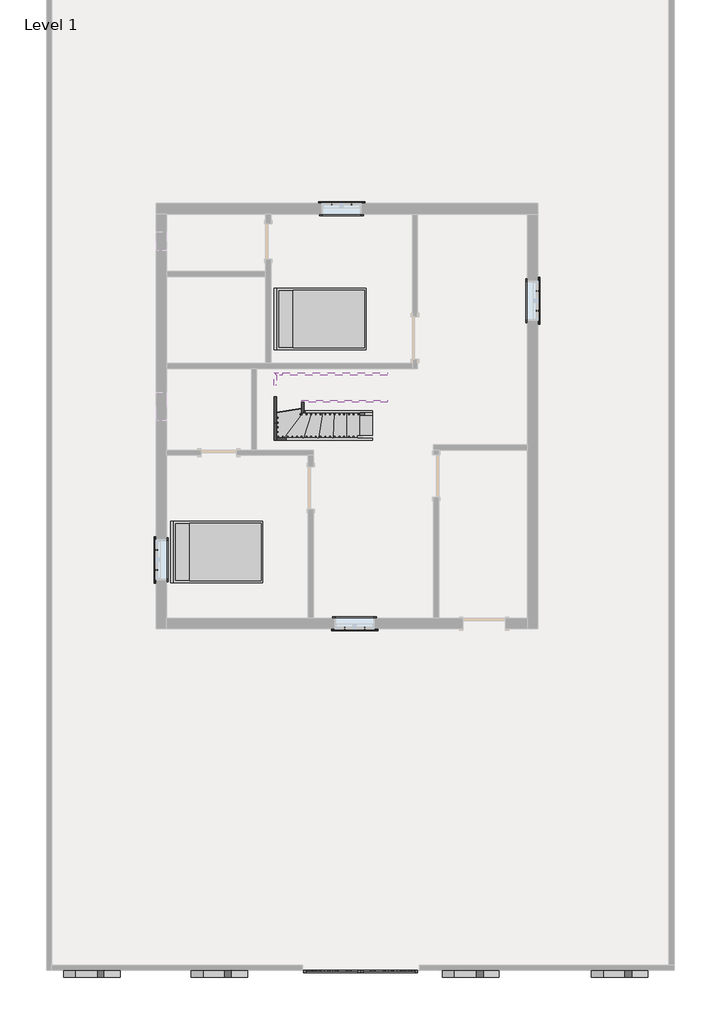
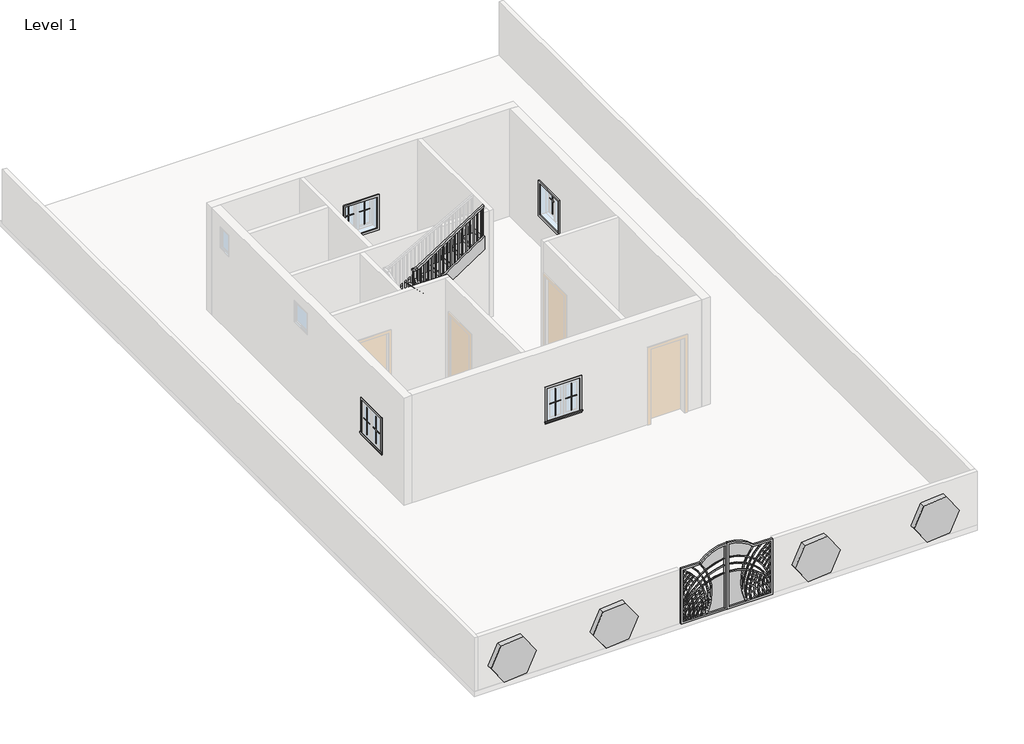
# One storey, part 2 of 2: 18 proxies, 9 members, 2 furniture elements, 1 railing, 1 stair flight.
"""IFC4 building model written with IfcOpenShell, lengths in millimetres."""

from ifc_helpers import new_model, si_unit, frame, origin, place, context, project, spatial, polyline, outline, extrude, faceted_brep, transform, mapped, element, save
from components import generic_models_6bc30956, generic_models_1_generic_models_1_2c748ff4, muntin_pattern_2x2_muntin_pattern_2x2_b3fe6957, muntin_pattern_2x2_muntin_pattern_2x2_3e0ecaf2, trim_window_exterior_flat_with_sill_41619996, trim_window_interior_flat_picture_frame_51c85655, bed_17739_bed_17739_15c61121, stair_flight_0735e5f0

model = new_model("IFC4")

# Units and contexts
model_context = context("Model", 3, world=origin())
ifc_project = project(units=[si_unit("LENGTHUNIT", "METRE", prefix="MILLI")], contexts=[model_context])

# Site, building, storey
site = spatial("IfcSite", under=ifc_project)
building = spatial("IfcBuilding", under=site)
storey = spatial("IfcBuildingStorey", under=building, Name="Level 1", Elevation=0.0)

# Proxies
placement = place(None, origin())
generic_models_shape = generic_models_6bc30956(model_context)
element("IfcBuildingElementProxy", 1, Name="Generic Models", at=placement, inside=storey, context=model_context, shape_type="MappedRepresentation", body=[
    mapped(generic_models_shape, transform((-524.3667921, -11737.015504, 0.0), x_axis=(1.0, 0.0, 0.0), y_axis=(0.0, 1.0, 0.0), z_axis=(0.0, 0.0, 1.0))),
])
generic_models_1_generic_models_1_shape = generic_models_1_generic_models_1_2c748ff4(model_context)
element("IfcBuildingElementProxy", 2, Name="Generic Models 1 : Generic Models 1", ObjectType="Generic Models 1 : Generic Models 1", at=placement, inside=storey, context=model_context, shape_type="MappedRepresentation", body=[
    mapped(generic_models_1_generic_models_1_shape, transform((0.0, 0.0, 0.0), x_axis=(1.0, 0.0, 0.0), y_axis=(0.0, 1.0, 0.0), z_axis=(0.0, 0.0, 1.0))),
])
muntin_pattern_2x2_muntin_pattern_2x2_shape = muntin_pattern_2x2_muntin_pattern_2x2_b3fe6957(model_context)
element("IfcBuildingElementProxy", 3, Name="Muntin Pattern_2x2 : Muntin Pattern_2x2", ObjectType="Muntin Pattern_2x2 : Muntin Pattern_2x2", at=placement, inside=storey, context=model_context, shape_type="MappedRepresentation", body=[
    mapped(muntin_pattern_2x2_muntin_pattern_2x2_shape, transform((-1143.3273498, 4766.5933073, 984.25), x_axis=(1.0, 0.0, 0.0), y_axis=(0.0, 1.0, 0.0), z_axis=(0.0, 0.0, 1.0))),
])
element("IfcBuildingElementProxy", 4, Name="Muntin Pattern_2x2 : Muntin Pattern_2x2", ObjectType="Muntin Pattern_2x2 : Muntin Pattern_2x2", at=placement, inside=storey, context=model_context, shape_type="MappedRepresentation", body=[
    mapped(muntin_pattern_2x2_muntin_pattern_2x2_shape, transform((3290.5601502, 2894.9308073, 984.25), x_axis=(0.0, -1.0, 0.0), y_axis=(1.0, 0.0, 0.0), z_axis=(0.0, 0.0, 1.0))),
])
element("IfcBuildingElementProxy", 5, Name="Muntin Pattern_2x2 : Muntin Pattern_2x2", ObjectType="Muntin Pattern_2x2 : Muntin Pattern_2x2", at=placement, inside=storey, context=model_context, shape_type="MappedRepresentation", body=[
    mapped(muntin_pattern_2x2_muntin_pattern_2x2_shape, transform((-4919.9898498, -3112.1691927, 984.25), x_axis=(0.0, 1.0, 0.0), y_axis=(-1.0, 0.0, 0.0), z_axis=(0.0, 0.0, 1.0))),
])
element("IfcBuildingElementProxy", 6, Name="Muntin Pattern_2x2 : Muntin Pattern_2x2", ObjectType="Muntin Pattern_2x2 : Muntin Pattern_2x2", at=placement, inside=storey, context=model_context, shape_type="MappedRepresentation", body=[
    mapped(muntin_pattern_2x2_muntin_pattern_2x2_shape, transform((-433.8792921, -4374.2316927, 1136.65), x_axis=(-1.0, 0.0, 0.0), y_axis=(0.0, -1.0, 0.0), z_axis=(0.0, 0.0, 1.0))),
])
muntin_pattern_2x2_muntin_pattern_2x2_2_shape = muntin_pattern_2x2_muntin_pattern_2x2_3e0ecaf2(model_context)
element("IfcBuildingElementProxy", 7, Name="Muntin Pattern_2x2 : Muntin Pattern_2x2", ObjectType="Muntin Pattern_2x2 : Muntin Pattern_2x2", at=placement, inside=storey, context=model_context, shape_type="MappedRepresentation", body=[
    mapped(muntin_pattern_2x2_muntin_pattern_2x2_2_shape, transform((-714.7023498, 4766.5933073, 984.25), x_axis=(-1.0, 0.0, 0.0), y_axis=(0.0, -1.0, 0.0), z_axis=(0.0, 0.0, 1.0))),
])
element("IfcBuildingElementProxy", 8, Name="Muntin Pattern_2x2 : Muntin Pattern_2x2", ObjectType="Muntin Pattern_2x2 : Muntin Pattern_2x2", at=placement, inside=storey, context=model_context, shape_type="MappedRepresentation", body=[
    mapped(muntin_pattern_2x2_muntin_pattern_2x2_2_shape, transform((3290.5601502, 2466.3058073, 984.25), x_axis=(0.0, 1.0, 0.0), y_axis=(-1.0, 0.0, 0.0), z_axis=(0.0, 0.0, 1.0))),
])
element("IfcBuildingElementProxy", 9, Name="Muntin Pattern_2x2 : Muntin Pattern_2x2", ObjectType="Muntin Pattern_2x2 : Muntin Pattern_2x2", at=placement, inside=storey, context=model_context, shape_type="MappedRepresentation", body=[
    mapped(muntin_pattern_2x2_muntin_pattern_2x2_2_shape, transform((-4919.9898498, -2683.5441927, 984.25), x_axis=(0.0, -1.0, 0.0), y_axis=(1.0, 0.0, 0.0), z_axis=(0.0, 0.0, 1.0))),
])
element("IfcBuildingElementProxy", 10, Name="Muntin Pattern_2x2 : Muntin Pattern_2x2", ObjectType="Muntin Pattern_2x2 : Muntin Pattern_2x2", at=placement, inside=storey, context=model_context, shape_type="MappedRepresentation", body=[
    mapped(muntin_pattern_2x2_muntin_pattern_2x2_2_shape, transform((-862.5042921, -4374.2316927, 1136.65), x_axis=(1.0, 0.0, 0.0), y_axis=(0.0, 1.0, 0.0), z_axis=(0.0, 0.0, 1.0))),
])
trim_window_exterior_flat_with_sill_shape = trim_window_exterior_flat_with_sill_41619996(model_context)
element("IfcBuildingElementProxy", 11, Name="Trim-Window-Exterior-Flat : with Sill", ObjectType="Trim-Window-Exterior-Flat : with Sill", at=placement, inside=storey, context=model_context, shape_type="MappedRepresentation", body=[
    mapped(trim_window_exterior_flat_with_sill_shape, transform((-929.0148498, 4776.1183073, 1828.8), x_axis=(-1.0, 0.0, 0.0), y_axis=(0.0, 0.0, 1.0), z_axis=(0.0, 1.0, 0.0))),
])
element("IfcBuildingElementProxy", 12, Name="Trim-Window-Exterior-Flat : with Sill", ObjectType="Trim-Window-Exterior-Flat : with Sill", at=placement, inside=storey, context=model_context, shape_type="MappedRepresentation", body=[
    mapped(trim_window_exterior_flat_with_sill_shape, transform((3300.0851502, 2680.6183073, 1828.8), x_axis=(0.0, 1.0, 0.0), y_axis=(0.0, 0.0, 1.0), z_axis=(1.0, 0.0, 0.0))),
])
element("IfcBuildingElementProxy", 13, Name="Trim-Window-Exterior-Flat : with Sill", ObjectType="Trim-Window-Exterior-Flat : with Sill", at=placement, inside=storey, context=model_context, shape_type="MappedRepresentation", body=[
    mapped(trim_window_exterior_flat_with_sill_shape, transform((-4929.5148498, -2897.8566927, 1828.8), x_axis=(0.0, -1.0, 0.0), y_axis=(0.0, 0.0, 1.0), z_axis=(-1.0, 0.0, 0.0))),
])
element("IfcBuildingElementProxy", 14, Name="Trim-Window-Exterior-Flat : with Sill", ObjectType="Trim-Window-Exterior-Flat : with Sill", at=placement, inside=storey, context=model_context, shape_type="MappedRepresentation", body=[
    mapped(trim_window_exterior_flat_with_sill_shape, transform((-648.1917921, -4383.7566927, 1981.2), x_axis=(1.0, 0.0, 0.0), y_axis=(0.0, 0.0, 1.0), z_axis=(0.0, -1.0, 0.0))),
])
trim_window_interior_flat_picture_frame_shape = trim_window_interior_flat_picture_frame_51c85655(model_context)
element("IfcBuildingElementProxy", 15, Name="Trim-Window-Interior-Flat : Picture Frame", ObjectType="Trim-Window-Interior-Flat : Picture Frame", at=placement, inside=storey, context=model_context, shape_type="MappedRepresentation", body=[
    mapped(trim_window_interior_flat_picture_frame_shape, transform((-929.0148498, 4547.5183073, 1828.8), x_axis=(1.0, 0.0, 0.0), y_axis=(0.0, 0.0, 1.0), z_axis=(0.0, -1.0, 0.0))),
])
element("IfcBuildingElementProxy", 16, Name="Trim-Window-Interior-Flat : Picture Frame", ObjectType="Trim-Window-Interior-Flat : Picture Frame", at=placement, inside=storey, context=model_context, shape_type="MappedRepresentation", body=[
    mapped(trim_window_interior_flat_picture_frame_shape, transform((3071.4851502, 2680.6183073, 1828.8), x_axis=(0.0, -1.0, 0.0), y_axis=(0.0, 0.0, 1.0), z_axis=(-1.0, 0.0, 0.0))),
])
element("IfcBuildingElementProxy", 17, Name="Trim-Window-Interior-Flat : Picture Frame", ObjectType="Trim-Window-Interior-Flat : Picture Frame", at=placement, inside=storey, context=model_context, shape_type="MappedRepresentation", body=[
    mapped(trim_window_interior_flat_picture_frame_shape, transform((-4700.9148498, -2897.8566927, 1828.8), x_axis=(0.0, 1.0, 0.0), y_axis=(0.0, 0.0, 1.0), z_axis=(1.0, 0.0, 0.0))),
])
element("IfcBuildingElementProxy", 18, Name="Trim-Window-Interior-Flat : Picture Frame", ObjectType="Trim-Window-Interior-Flat : Picture Frame", at=placement, inside=storey, context=model_context, shape_type="MappedRepresentation", body=[
    mapped(trim_window_interior_flat_picture_frame_shape, transform((-648.1917921, -4155.1566927, 1981.2), x_axis=(-1.0, 0.0, 0.0), y_axis=(0.0, 0.0, 1.0), z_axis=(0.0, 1.0, 0.0))),
])

# Furniture
bed_17739_bed_17739_shape = bed_17739_bed_17739_15c61121(model_context)
element("IfcFurniture", 19, ObjectType="Bed_17739 : Bed_17739", at=placement, inside=storey, context=model_context, shape_type="MappedRepresentation", body=[
    mapped(bed_17739_bed_17739_shape, transform((-3596.0148498, -2726.4066927, 0.0), x_axis=(0.0, 1.0, 0.0), y_axis=(-1.0, 0.0, 0.0), z_axis=(0.0, 0.0, 1.0))),
])
element("IfcFurniture", 20, ObjectType="Bed_17739 : Bed_17739", at=placement, inside=storey, context=model_context, shape_type="MappedRepresentation", body=[
    mapped(bed_17739_bed_17739_shape, transform((-1367.1648498, 2290.0933073, 0.0), x_axis=(0.0, 1.0, 0.0), y_axis=(-1.0, 0.0, 0.0), z_axis=(0.0, 0.0, 1.0))),
])

# Members
element("IfcMember", 21, ObjectType="Stringer - 2\" Width", at=placement, inside=storey, context=model_context, shape_type="SweptSolid", body=[
    extrude(outline(polyline([(0.0, -264.8831579), (228.4652135, -264.8831579), (1304.2576628, -2328.8610857), (960.5393024, -2328.8610857), (0.0, -486.0038318), (0.0, -264.8831579)])), frame((0.0, -322.6029286, 0.0), z_axis=(0.0, 1.0, 0.0), x_axis=(0.0, 0.0, 1.0)), (0.0, 0.0, 1.0), 50.8),
])
element("IfcMember", 22, ObjectType="Stringer - 2\" Width", at=placement, inside=storey, context=model_context, shape_type="SweptSolid", body=[
    extrude(outline(polyline([(-2328.8610857, -322.6029286), (-2379.6610857, -322.6029286), (-2379.6610857, 39.7116887), (-2328.8610857, 39.7116887), (-2328.8610857, -322.6029286)])), frame((0.0, 0.0, 960.5393024), z_axis=(0.0, 0.0, 1.0), x_axis=(1.0, 0.0, 0.0)), (0.0, 0.0, 1.0), 343.7183604),
])
element("IfcMember", 23, ObjectType="Stringer - 2\" Width", at=placement, inside=storey, context=model_context, shape_type="SweptSolid", body=[
    extrude(outline(polyline([(39.7116887, 960.5393024), (39.7116887, 1304.2576628), (861.172384, 1644.0948766), (861.172384, 1300.3765162), (39.7116887, 960.5393024)])), frame((-2379.6610857, 0.0, 0.0), z_axis=(1.0, 0.0, 0.0), x_axis=(0.0, 1.0, 0.0)), (0.0, 0.0, 1.0), 50.8),
])
element("IfcMember", 24, ObjectType="Stringer - 2\" Width", at=placement, inside=storey, context=model_context, shape_type="SweptSolid", body=[
    extrude(outline(polyline([(-2328.8610857, 861.172384), (-2379.6610857, 861.172384), (-2379.6610857, 1130.8895433), (-2328.8610857, 1080.0895433), (-2328.8610857, 861.172384)])), frame((0.0, 0.0, 1306.6790002), z_axis=(0.0, 0.0, 1.0), x_axis=(1.0, 0.0, 0.0)), (0.0, 0.0, 1.0), 329.8531189),
])
element("IfcMember", 25, ObjectType="Stringer - 2\" Width", at=placement, inside=storey, context=model_context, shape_type="SweptSolid", body=[
    extrude(outline(polyline([(-2328.8610857, 1080.0895433), (-2379.6610857, 1130.8895433), (-2203.9193363, 1130.8895433), (-2203.9193363, 1080.0895433), (-2328.8610857, 1080.0895433)])), frame((0.0, 0.0, 1306.6790002), z_axis=(0.0, 0.0, 1.0), x_axis=(1.0, 0.0, 0.0)), (0.0, 0.0, 1.0), 329.8531189),
])
element("IfcMember", 26, ObjectType="Stringer - 2\" Width", at=placement, inside=storey, context=model_context, shape_type="SweptSolid", body=[
    extrude(outline(polyline([(0.0, -264.8831579), (196.9581828, -264.8831579), (1216.4545254, -1741.8148498), (846.0897368, -1741.8148498), (0.0, -516.0951544), (0.0, -264.8831579)])), frame((0.0, 264.4433073, 0.0), z_axis=(0.0, 1.0, 0.0), x_axis=(0.0, 0.0, 1.0)), (0.0, 0.0, 1.0), 50.8),
])
element("IfcMember", 27, ObjectType="Stringer - 2\" Width", at=placement, inside=storey, context=model_context, shape_type="SweptSolid", body=[
    extrude(outline(polyline([(264.4433073, 925.7590756), (264.4433073, 1384.958282), (493.0433073, 1642.5490234), (493.0433073, 1183.349817), (264.4433073, 925.7590756)])), frame((-1792.6148498, 0.0, 0.0), z_axis=(1.0, 0.0, 0.0), x_axis=(0.0, 1.0, 0.0)), (0.0, 0.0, 1.0), 50.8),
])
element("IfcMember", 28, ObjectType="Stringer - 2\" Width", at=placement, inside=storey, context=model_context, shape_type="SweptSolid", body=[
    extrude(outline(polyline([(1715.6438732, -1792.6148498), (1350.3121415, -1792.6148498), (2576.7313098, 63.4034409), (2942.0630415, 63.4034409), (1715.6438732, -1792.6148498)])), frame((0.0, 493.0433073, 0.0), z_axis=(0.0, 1.0, 0.0), x_axis=(0.0, 0.0, 1.0)), (0.0, 0.0, 1.0), 50.8),
])
element("IfcMember", 29, ObjectType="Stringer - 2\" Width", at=placement, inside=storey, context=model_context, shape_type="SweptSolid", body=[
    extrude(outline(polyline([(1636.532119, -2203.9193363), (1306.6790002, -2203.9193363), (2562.042957, 63.4034409), (2891.8960758, 63.4034409), (1636.532119, -2203.9193363)])), frame((0.0, 1080.0895433, 0.0), z_axis=(0.0, 1.0, 0.0), x_axis=(0.0, 0.0, 1.0)), (0.0, 0.0, 1.0), 50.8),
])

# Railing
element("IfcRailing", 30, ObjectType="Handrail - Rectangular", at=placement, inside=storey, context=model_context, shape_type="SolidModel", body=[
    faceted_brep([(-264.8831579, 213.6433073, 1083.7333333), (-264.8831579, 213.6433073, 1022.4533076), (-264.8831579, 264.4433073, 1022.4533076), (-264.8831579, 264.4433073, 1083.7333333), (-1716.4148498, 213.6433073, 2063.0160626), (-1767.2148498, 213.6433073, 2036.0084974), (-1767.2148498, 264.4433073, 2036.0084974), (-1716.4148498, 264.4433073, 2063.0160626), (-1716.4148498, 213.6433073, 2277.5989826), (-1767.2148498, 213.6433073, 2226.7989826), (-1767.2148498, 264.4433073, 2226.7989826), (-1716.4148498, 264.4433073, 2277.5989826), (-1843.4148498, 213.6433073, 2277.5989826), (-1843.4148498, 213.6433073, 2226.7989826), (-1792.6148498, 264.4433073, 2226.7989826), (-1792.6148498, 264.4433073, 2277.5989826), (-1843.4148498, 340.6433073, 2277.5989826), (-1843.4148498, 363.4803462, 2226.7989826), (-1792.6148498, 363.4803462, 2226.7989826), (-1792.6148498, 340.6433073, 2277.5989826), (-1843.4148498, 467.6433073, 2420.70495), (-1843.4148498, 518.4433073, 2401.4141359), (-1792.6148498, 518.4433073, 2401.4141359), (-1792.6148498, 467.6433073, 2420.70495), (-1843.4148498, 467.6433073, 2631.974751), (-1843.4148498, 518.4433073, 2581.174751), (-1792.6148498, 518.4433073, 2581.174751), (-1792.6148498, 467.6433073, 2631.974751), (-1843.4148498, 594.6433073, 2631.974751), (-1843.4148498, 594.6433073, 2581.174751), (-1792.6148498, 543.8433073, 2581.174751), (-1792.6148498, 543.8433073, 2631.974751), (-1716.4148498, 594.6433073, 2631.974751), (-1701.3097842, 594.6433073, 2581.174751), (-1701.3097842, 543.8433073, 2581.174751), (-1716.4148498, 543.8433073, 2631.974751), (63.4034409, 594.6433073, 3793.0666667), (63.4034409, 543.8433073, 3793.0666667), (63.4034409, 543.8433073, 3732.4126442), (63.4034409, 594.6433073, 3732.4126442)], [[[0, 1, 2, 3]], [[1, 0, 4, 5]], [[2, 1, 5, 6]], [[3, 2, 6, 7]], [[0, 3, 7, 4]], [[5, 4, 8, 9]], [[6, 5, 9, 10]], [[7, 6, 10, 11]], [[4, 7, 11, 8]], [[9, 8, 12, 13]], [[10, 9, 13, 14]], [[11, 10, 14, 15]], [[8, 11, 15, 12]], [[13, 12, 16, 17]], [[14, 13, 17, 18]], [[15, 14, 18, 19]], [[12, 15, 19, 16]], [[17, 16, 20, 21]], [[18, 17, 21, 22]], [[19, 18, 22, 23]], [[16, 19, 23, 20]], [[21, 20, 24, 25]], [[22, 21, 25, 26]], [[23, 22, 26, 27]], [[20, 23, 27, 24]], [[25, 24, 28, 29]], [[26, 25, 29, 30]], [[27, 26, 30, 31]], [[24, 27, 31, 28]], [[29, 28, 32, 33]], [[30, 29, 33, 34]], [[31, 30, 34, 35]], [[28, 31, 35, 32]], [[36, 37, 38, 39]], [[33, 32, 36, 39]], [[34, 33, 39, 38]], [[35, 34, 38, 37]], [[32, 35, 37, 36]]]),
    extrude(outline(polyline([(3704.3000713, 20.3101502), (3691.87251, 1.2601502), (2709.3333333, 1.2601502), (2709.3333333, 20.3101502), (3704.3000713, 20.3101502)])), frame((0.0, 559.7183073, 0.0), z_axis=(0.0, 1.0, 0.0), x_axis=(0.0, 0.0, 1.0)), (0.0, 0.0, 1.0), 19.05),
    extrude(outline(polyline([(3638.0197441, -81.2898498), (3625.5921828, -100.3398498), (2709.3333333, -100.3398498), (2709.3333333, -81.2898498), (3638.0197441, -81.2898498)])), frame((0.0, 559.7183073, 0.0), z_axis=(0.0, 1.0, 0.0), x_axis=(0.0, 0.0, 1.0)), (0.0, 0.0, 1.0), 19.05),
    extrude(outline(polyline([(3571.739417, -182.8898498), (3559.3118556, -201.9398498), (2709.3333333, -201.9398498), (2709.3333333, -182.8898498), (3571.739417, -182.8898498)])), frame((0.0, 559.7183073, 0.0), z_axis=(0.0, 1.0, 0.0), x_axis=(0.0, 0.0, 1.0)), (0.0, 0.0, 1.0), 19.05),
    extrude(outline(polyline([(3505.4590898, -284.4898498), (3493.0315284, -303.5398498), (2540.0, -303.5398498), (2540.0, -284.4898498), (3505.4590898, -284.4898498)])), frame((0.0, 559.7183073, 0.0), z_axis=(0.0, 1.0, 0.0), x_axis=(0.0, 0.0, 1.0)), (0.0, 0.0, 1.0), 19.05),
    extrude(outline(polyline([(3439.1787626, -386.0898498), (3426.7512013, -405.1398498), (2540.0, -405.1398498), (2540.0, -386.0898498), (3439.1787626, -386.0898498)])), frame((0.0, 559.7183073, 0.0), z_axis=(0.0, 1.0, 0.0), x_axis=(0.0, 0.0, 1.0)), (0.0, 0.0, 1.0), 19.05),
    extrude(outline(polyline([(3372.8984354, -487.6898498), (3360.4708741, -506.7398498), (2370.6666667, -506.7398498), (2370.6666667, -487.6898498), (3372.8984354, -487.6898498)])), frame((0.0, 559.7183073, 0.0), z_axis=(0.0, 1.0, 0.0), x_axis=(0.0, 0.0, 1.0)), (0.0, 0.0, 1.0), 19.05),
    extrude(outline(polyline([(3306.6181082, -589.2898498), (3294.1905469, -608.3398498), (2370.6666667, -608.3398498), (2370.6666667, -589.2898498), (3306.6181082, -589.2898498)])), frame((0.0, 559.7183073, 0.0), z_axis=(0.0, 1.0, 0.0), x_axis=(0.0, 0.0, 1.0)), (0.0, 0.0, 1.0), 19.05),
    extrude(outline(polyline([(3240.3377811, -690.8898498), (3227.9102197, -709.9398498), (2370.6666667, -709.9398498), (2370.6666667, -690.8898498), (3240.3377811, -690.8898498)])), frame((0.0, 559.7183073, 0.0), z_axis=(0.0, 1.0, 0.0), x_axis=(0.0, 0.0, 1.0)), (0.0, 0.0, 1.0), 19.05),
    extrude(outline(polyline([(3174.0574539, -792.4898498), (3161.6298925, -811.5398498), (2201.3333333, -811.5398498), (2201.3333333, -792.4898498), (3174.0574539, -792.4898498)])), frame((0.0, 559.7183073, 0.0), z_axis=(0.0, 1.0, 0.0), x_axis=(0.0, 0.0, 1.0)), (0.0, 0.0, 1.0), 19.05),
    extrude(outline(polyline([(3107.7771267, -894.0898498), (3095.3495653, -913.1398498), (2201.3333333, -913.1398498), (2201.3333333, -894.0898498), (3107.7771267, -894.0898498)])), frame((0.0, 559.7183073, 0.0), z_axis=(0.0, 1.0, 0.0), x_axis=(0.0, 0.0, 1.0)), (0.0, 0.0, 1.0), 19.05),
    extrude(outline(polyline([(3041.4967995, -995.6898498), (3029.0692382, -1014.7398498), (2201.3333333, -1014.7398498), (2201.3333333, -995.6898498), (3041.4967995, -995.6898498)])), frame((0.0, 559.7183073, 0.0), z_axis=(0.0, 1.0, 0.0), x_axis=(0.0, 0.0, 1.0)), (0.0, 0.0, 1.0), 19.05),
    extrude(outline(polyline([(2975.2164723, -1097.2898498), (2962.788911, -1116.3398498), (2032.0, -1116.3398498), (2032.0, -1097.2898498), (2975.2164723, -1097.2898498)])), frame((0.0, 559.7183073, 0.0), z_axis=(0.0, 1.0, 0.0), x_axis=(0.0, 0.0, 1.0)), (0.0, 0.0, 1.0), 19.05),
    extrude(outline(polyline([(2908.9361451, -1198.8898498), (2896.5085838, -1217.9398498), (2032.0, -1217.9398498), (2032.0, -1198.8898498), (2908.9361451, -1198.8898498)])), frame((0.0, 559.7183073, 0.0), z_axis=(0.0, 1.0, 0.0), x_axis=(0.0, 0.0, 1.0)), (0.0, 0.0, 1.0), 19.05),
    extrude(outline(polyline([(2842.655818, -1300.4898498), (2830.2282566, -1319.5398498), (1862.6666667, -1319.5398498), (1862.6666667, -1300.4898498), (2842.655818, -1300.4898498)])), frame((0.0, 559.7183073, 0.0), z_axis=(0.0, 1.0, 0.0), x_axis=(0.0, 0.0, 1.0)), (0.0, 0.0, 1.0), 19.05),
    extrude(outline(polyline([(2776.3754908, -1402.0898498), (2763.9479294, -1421.1398498), (1862.6666667, -1421.1398498), (1862.6666667, -1402.0898498), (2776.3754908, -1402.0898498)])), frame((0.0, 559.7183073, 0.0), z_axis=(0.0, 1.0, 0.0), x_axis=(0.0, 0.0, 1.0)), (0.0, 0.0, 1.0), 19.05),
    extrude(outline(polyline([(2710.0951636, -1503.6898498), (2697.6676023, -1522.7398498), (1862.6666667, -1522.7398498), (1862.6666667, -1503.6898498), (2710.0951636, -1503.6898498)])), frame((0.0, 559.7183073, 0.0), z_axis=(0.0, 1.0, 0.0), x_axis=(0.0, 0.0, 1.0)), (0.0, 0.0, 1.0), 19.05),
    extrude(outline(polyline([(2643.8148364, -1605.2898498), (2631.3872751, -1624.3398498), (1693.3333333, -1624.3398498), (1693.3333333, -1605.2898498), (2643.8148364, -1605.2898498)])), frame((0.0, 559.7183073, 0.0), z_axis=(0.0, 1.0, 0.0), x_axis=(0.0, 0.0, 1.0)), (0.0, 0.0, 1.0), 19.05),
    extrude(outline(polyline([(2577.5345092, -1706.8898498), (2565.1069479, -1725.9398498), (1693.3333333, -1725.9398498), (1693.3333333, -1706.8898498), (2577.5345092, -1706.8898498)])), frame((0.0, 559.7183073, 0.0), z_axis=(0.0, 1.0, 0.0), x_axis=(0.0, 0.0, 1.0)), (0.0, 0.0, 1.0), 19.05),
    extrude(outline(polyline([(-1808.4898498, 534.3183073), (-1827.5398498, 534.3183073), (-1827.5398498, 553.3683073), (-1808.4898498, 553.3683073), (-1808.4898498, 534.3183073)])), frame((0.0, 0.0, 1524.0), z_axis=(0.0, 0.0, 1.0), x_axis=(1.0, 0.0, 0.0)), (0.0, 0.0, 1.0), 1057.174751),
    extrude(outline(polyline([(432.7183073, 2304.8176079), (451.7683073, 2326.283503), (451.7683073, 1354.6666667), (432.7183073, 1354.6666667), (432.7183073, 2304.8176079)])), frame((-1827.5398498, 0.0, 0.0), z_axis=(1.0, 0.0, 0.0), x_axis=(0.0, 1.0, 0.0)), (0.0, 0.0, 1.0), 19.05),
    extrude(outline(polyline([(331.1183073, 2190.332834), (350.1683073, 2211.7987291), (350.1683073, 1354.6666667), (331.1183073, 1354.6666667), (331.1183073, 2190.332834)])), frame((-1827.5398498, 0.0, 0.0), z_axis=(1.0, 0.0, 0.0), x_axis=(0.0, 1.0, 0.0)), (0.0, 0.0, 1.0), 19.05),
    extrude(outline(polyline([(-1779.3581579, 248.5683073), (-1779.3581579, 229.5183073), (-1798.4081579, 229.5183073), (-1798.4081579, 248.5683073), (-1779.3581579, 248.5683073)])), frame((0.0, 0.0, 1016.0), z_axis=(0.0, 0.0, 1.0), x_axis=(1.0, 0.0, 0.0)), (0.0, 0.0, 1.0), 1210.7989826),
    extrude(outline(polyline([(1975.6561166, -1677.7581579), (1988.5082893, -1696.8081579), (1016.0, -1696.8081579), (1016.0, -1677.7581579), (1975.6561166, -1677.7581579)])), frame((0.0, 229.5183073, 0.0), z_axis=(0.0, 1.0, 0.0), x_axis=(0.0, 0.0, 1.0)), (0.0, 0.0, 1.0), 19.05),
    extrude(outline(polyline([(1907.1111955, -1576.1581579), (1919.9633682, -1595.2081579), (1016.0, -1595.2081579), (1016.0, -1576.1581579), (1907.1111955, -1576.1581579)])), frame((0.0, 229.5183073, 0.0), z_axis=(0.0, 1.0, 0.0), x_axis=(0.0, 0.0, 1.0)), (0.0, 0.0, 1.0), 19.05),
    extrude(outline(polyline([(1838.5662744, -1474.5581579), (1851.4184472, -1493.6081579), (846.6666667, -1493.6081579), (846.6666667, -1474.5581579), (1838.5662744, -1474.5581579)])), frame((0.0, 229.5183073, 0.0), z_axis=(0.0, 1.0, 0.0), x_axis=(0.0, 0.0, 1.0)), (0.0, 0.0, 1.0), 19.05),
    extrude(outline(polyline([(1770.0213533, -1372.9581579), (1782.8735261, -1392.0081579), (846.6666667, -1392.0081579), (846.6666667, -1372.9581579), (1770.0213533, -1372.9581579)])), frame((0.0, 229.5183073, 0.0), z_axis=(0.0, 1.0, 0.0), x_axis=(0.0, 0.0, 1.0)), (0.0, 0.0, 1.0), 19.05),
    extrude(outline(polyline([(1701.4764322, -1271.3581579), (1714.328605, -1290.4081579), (677.3333333, -1290.4081579), (677.3333333, -1271.3581579), (1701.4764322, -1271.3581579)])), frame((0.0, 229.5183073, 0.0), z_axis=(0.0, 1.0, 0.0), x_axis=(0.0, 0.0, 1.0)), (0.0, 0.0, 1.0), 19.05),
    extrude(outline(polyline([(1632.9315111, -1169.7581579), (1645.7836839, -1188.8081579), (677.3333333, -1188.8081579), (677.3333333, -1169.7581579), (1632.9315111, -1169.7581579)])), frame((0.0, 229.5183073, 0.0), z_axis=(0.0, 1.0, 0.0), x_axis=(0.0, 0.0, 1.0)), (0.0, 0.0, 1.0), 19.05),
    extrude(outline(polyline([(1564.3865901, -1068.1581579), (1577.2387628, -1087.2081579), (508.0, -1087.2081579), (508.0, -1068.1581579), (1564.3865901, -1068.1581579)])), frame((0.0, 229.5183073, 0.0), z_axis=(0.0, 1.0, 0.0), x_axis=(0.0, 0.0, 1.0)), (0.0, 0.0, 1.0), 19.05),
    extrude(outline(polyline([(1495.841669, -966.5581579), (1508.6938417, -985.6081579), (508.0, -985.6081579), (508.0, -966.5581579), (1495.841669, -966.5581579)])), frame((0.0, 229.5183073, 0.0), z_axis=(0.0, 1.0, 0.0), x_axis=(0.0, 0.0, 1.0)), (0.0, 0.0, 1.0), 19.05),
    extrude(outline(polyline([(1427.2967479, -864.9581579), (1440.1489206, -884.0081579), (508.0, -884.0081579), (508.0, -864.9581579), (1427.2967479, -864.9581579)])), frame((0.0, 229.5183073, 0.0), z_axis=(0.0, 1.0, 0.0), x_axis=(0.0, 0.0, 1.0)), (0.0, 0.0, 1.0), 19.05),
    extrude(outline(polyline([(1358.7518268, -763.3581579), (1371.6039995, -782.4081579), (338.6666667, -782.4081579), (338.6666667, -763.3581579), (1358.7518268, -763.3581579)])), frame((0.0, 229.5183073, 0.0), z_axis=(0.0, 1.0, 0.0), x_axis=(0.0, 0.0, 1.0)), (0.0, 0.0, 1.0), 19.05),
    extrude(outline(polyline([(1290.2069057, -661.7581579), (1303.0590784, -680.8081579), (338.6666667, -680.8081579), (338.6666667, -661.7581579), (1290.2069057, -661.7581579)])), frame((0.0, 229.5183073, 0.0), z_axis=(0.0, 1.0, 0.0), x_axis=(0.0, 0.0, 1.0)), (0.0, 0.0, 1.0), 19.05),
    extrude(outline(polyline([(1221.6619846, -560.1581579), (1234.5141573, -579.2081579), (338.6666667, -579.2081579), (338.6666667, -560.1581579), (1221.6619846, -560.1581579)])), frame((0.0, 229.5183073, 0.0), z_axis=(0.0, 1.0, 0.0), x_axis=(0.0, 0.0, 1.0)), (0.0, 0.0, 1.0), 19.05),
    extrude(outline(polyline([(1153.1170635, -458.5581579), (1165.9692362, -477.6081579), (169.3333333, -477.6081579), (169.3333333, -458.5581579), (1153.1170635, -458.5581579)])), frame((0.0, 229.5183073, 0.0), z_axis=(0.0, 1.0, 0.0), x_axis=(0.0, 0.0, 1.0)), (0.0, 0.0, 1.0), 19.05),
    extrude(outline(polyline([(1084.5721424, -356.9581579), (1097.4243151, -376.0081579), (169.3333333, -376.0081579), (169.3333333, -356.9581579), (1084.5721424, -356.9581579)])), frame((0.0, 229.5183073, 0.0), z_axis=(0.0, 1.0, 0.0), x_axis=(0.0, 0.0, 1.0)), (0.0, 0.0, 1.0), 19.05),
    extrude(outline(polyline([(-1808.4898498, 559.7183073), (-1827.5398498, 559.7183073), (-1827.5398498, 578.7683073), (-1808.4898498, 578.7683073), (-1808.4898498, 559.7183073)])), frame((0.0, 0.0, 1524.0), z_axis=(0.0, 0.0, 1.0), x_axis=(1.0, 0.0, 0.0)), (0.0, 0.0, 1.0), 1057.174751),
    extrude(outline(polyline([(-1808.4898498, 248.5683073), (-1808.4898498, 229.5183073), (-1827.5398498, 229.5183073), (-1827.5398498, 248.5683073), (-1808.4898498, 248.5683073)])), frame((0.0, 0.0, 1185.3333333), z_axis=(0.0, 0.0, 1.0), x_axis=(1.0, 0.0, 0.0)), (0.0, 0.0, 1.0), 1041.4656493),
    extrude(outline(polyline([(3732.4126442, 63.4034409), (3719.9850828, 44.3534409), (2709.3333333, 44.3534409), (2709.3333333, 63.4034409), (3732.4126442, 63.4034409)])), frame((0.0, 559.7183073, 0.0), z_axis=(0.0, 1.0, 0.0), x_axis=(0.0, 0.0, 1.0)), (0.0, 0.0, 1.0), 19.05),
    extrude(outline(polyline([(1022.4533076, -264.8831579), (1035.3054803, -283.9331579), (169.3333333, -283.9331579), (169.3333333, -264.8831579), (1022.4533076, -264.8831579)])), frame((0.0, 229.5183073, 0.0), z_axis=(0.0, 1.0, 0.0), x_axis=(0.0, 0.0, 1.0)), (0.0, 0.0, 1.0), 19.05),
])

# Stair flight
stair_flight_shape = stair_flight_0735e5f0(model_context)
element("IfcStairFlight", 31, ObjectType="2\" Tread 1\" Nosing 1/4\" Riser", at=placement, inside=storey, context=model_context, shape_type="MappedRepresentation", body=[
    mapped(stair_flight_shape, transform((0.0, 0.0, 0.0), x_axis=(1.0, 0.0, 0.0), y_axis=(0.0, 1.0, 0.0), z_axis=(0.0, 0.0, 1.0))),
])

save(model, "model.ifc")

# Revit data of these elements
# Type
#   m.s. sheet = none
#   2" x2" pipe = none
#   1"x1"pipe = none
#   Default Elevation = 0
# Type "Muntin Pattern_2x2 : Muntin Pattern_2x2"
#   Width [instance default] = 4' - 0"
#   Thickness = 0' - 0 1/2"
#   Height [instance default] = 4' - 0"
#   Distance = 0' - 0 3/4"
#   Interior Material [instance default] = none
#   Exterior Material [instance default] = none
#   Default Elevation = 0
# Type "Trim-Window-Exterior-Flat : with Sill"
#   Trim Width = 0' - 2 1/4"
#   Trim Thickness_Picture Frame = 0' - 1 1/4"
#   Trim Thickness_with Sill = 0' - 0 3/4"
#   Sill Thickness = 0' - 1 1/4"
#   Opening Width [instance default] = 2' - 0"
#   Opening Height [instance default] = 3' - 0"
#   Default Elevation = 4' - 0"
#   Sill = yes
#   Picture Frame = no
#   Trim Material [instance default] = none
# Type "Trim-Window-Interior-Flat : Picture Frame"
#   Trim Thickness_Picture Frame = 0' - 1 1/4"
#   Trim Width = 0' - 2 1/4"
#   Trim Thickness_with Sill = 0' - 0 3/4"
#   Sill Thickness = 0' - 1 1/4"
#   Opening Width [instance default] = 2' - 0"
#   Opening Height [instance default] = 3' - 0"
#   Default Elevation = 4' - 0"
#   Sill = no
#   Picture Frame = yes
#   Trim Material [instance default] = none
# Type "Bed_17739 : Bed_17739"
#   Default Elevation = 0
# Type "Handrail - Rectangular"
#   Assembly Code = "C2010400"
#   built-in parameter 1008612 = 0.0416667 (stored number, unit not read)
#   built-in parameter 1008611 = 0.0416667 (stored number, unit not read)
#   built-in parameter 1008609 = 0.333333 (stored number, unit not read)
#   built-in parameter 1008604 = 0.166667 (stored number, unit not read)
#   built-in parameter 1008603 = 0.166667 (stored number, unit not read)
#   Railing Height = 3' - 0"
#   built-in parameter 1008630 = 2
#   built-in parameter 1008610 = 2
#   built-in parameter 1008618 = Baluster - Square : 3/4"
# Element 1 (IfcBuildingElementProxy)
#   Phase Created = New Construction
#   Materials on its faces: "r1"
# Element 2 (IfcBuildingElementProxy, "Generic Models 1 : Generic Models 1")
#   Phase Created = New Construction
#   Materials on its faces: "Parking Stripe"
# Elements 3, 4, 5, 6, 7, 8, 9, 10 (IfcBuildingElementProxy, "Muntin Pattern_2x2 : Muntin Pattern_2x2")
#   Width = 0' - 11 5/8"
#   Height = 2' - 6 1/2"
#   Interior Material = Wood - Stained
#   Exterior Material = Clad - White
#   Phase Created = New Construction
#   Materials on its faces: "Clad - White", "Wood - Stained"
# Elements 11, 12, 13, 14 (IfcBuildingElementProxy, "Trim-Window-Exterior-Flat : with Sill")
#   Opening Width = 2' - 10"
#   Opening Height = 3' - 0"
#   Trim Material = Clad - White
#   Phase Created = New Construction
#   Materials on its faces: "Clad - White"
# Elements 15, 16, 17, 18 (IfcBuildingElementProxy, "Trim-Window-Interior-Flat : Picture Frame")
#   Opening Width = 2' - 10"
#   Opening Height = 3' - 0"
#   Trim Material = Wood - Stained
#   Phase Created = New Construction
#   Materials on its faces: "Wood - Stained"
# Elements 19, 20 (IfcFurniture, "Bed_17739 : Bed_17739")
#   Phase Created = New Construction
#   Materials on its faces: "legs", "sheets", "bed frame", "Blanket"
# Elements 21, 22, 23, 24, 25, 26, 27, 28, 29 (IfcMember, "Stringer - 2\" Width")
#   Phase Created = New Construction
# Element 30 (IfcRailing, "Handrail - Rectangular")
#   Phase Created = New Construction
# Element 31 (IfcStairFlight, "2\" Tread 1\" Nosing 1/4\" Riser")
#   Phase Created = New Construction
# Materials
#   "r1": class "Generic", colour RGB 120 120 120, transparency 0, Cost = 0
#   "Parking Stripe": class "Paint", colour RGB 250 250 91, transparency 0, Cost = 0
#   "Clad - White": class "Wood", colour RGB 242 242 238, transparency 0, Cost = 0
#   "Wood - Stained": class "Wood", colour RGB 224 178 126, transparency 0, Cost = 0
#   "legs": colour RGB 90 73 37, transparency 0, Cost = 0
#   "sheets": colour RGB 200 195 176, transparency 0, Cost = 0
#   "bed frame": colour RGB 90 73 37, transparency 0, Cost = 0
#   "Blanket": class "System", colour RGB 59 0 1, transparency 0, Cost = 0
